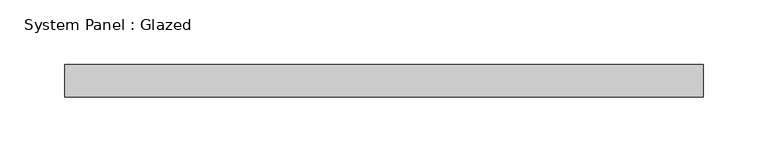
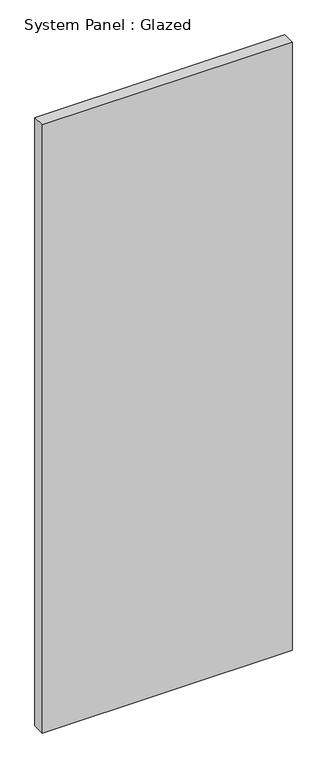
"""IFC4 building model written with IfcOpenShell, lengths in millimetres: plate geometry, System Panel : Glazed."""

from ifc_helpers import new_model, si_unit, origin, origin_with_axes, place, context, project, spatial, polyline, outline, extrude, source, transform, mapped, element, save


def system_panel_glazed_dc961f7d(model_context):
    return source(origin(), model_context, "Body", "SweptSolid", [
        extrude(outline(polyline([(247.65, 19.05), (-247.65, 19.05), (-247.65, 44.45), (247.65, 44.45), (247.65, 19.05)])), origin_with_axes(), (0.0, 0.0, 1.0), 1274.8499484),
    ])


if __name__ == "__main__":
    model = new_model("IFC4")
    model_context = context("Model", 3, world=origin())
    ifc_project = project(units=[si_unit("LENGTHUNIT", "METRE", prefix="MILLI")], contexts=[model_context])
    site = spatial("IfcSite", under=ifc_project)
    building = spatial("IfcBuilding", under=site)
    placement = place(None, origin())
    system_panel_glazed_shape = system_panel_glazed_dc961f7d(model_context)
    element("IfcPlate", 1, ObjectType="System Panel : Glazed", at=placement, inside=building, context=model_context, shape_type="MappedRepresentation", body=[
        mapped(system_panel_glazed_shape, transform((0.0, 0.0, 0.0), x_axis=(1.0, 0.0, 0.0), y_axis=(0.0, 1.0, 0.0), z_axis=(0.0, 0.0, 1.0))),
    ])
    save(model, "model.ifc")

# Revit data of these elements
# Type "System Panel : Glazed"
#   Construction Type Id = "GSP4R"
#   Analytic Construction = "1/8 in Pilkington single glazing"
#   Visual Light Transmittance = 0.9
#   Solar Heat Gain Coefficient = 0.86
#   Heat Transfer Coefficient (U) = 1.18115 BTU/(h·ft²·°F)
#   Define Thermal Properties by = 1
# Element 1 (IfcPlate, "System Panel : Glazed")
#   Materials on its faces: "Glass"
# Materials
#   "Glass": class "Glass", colour RGB 0 128 192, transparency 0.75, Description = "Soda Lime Glass", Cost = 0
